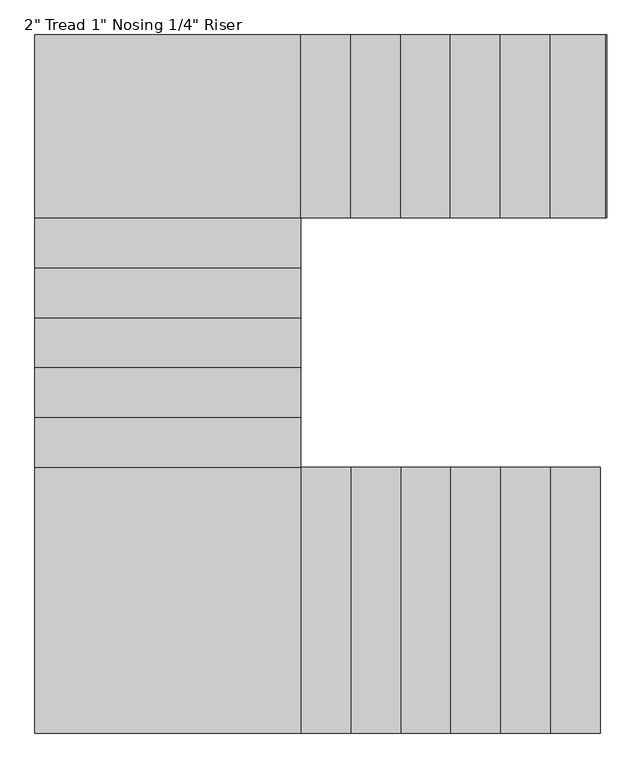
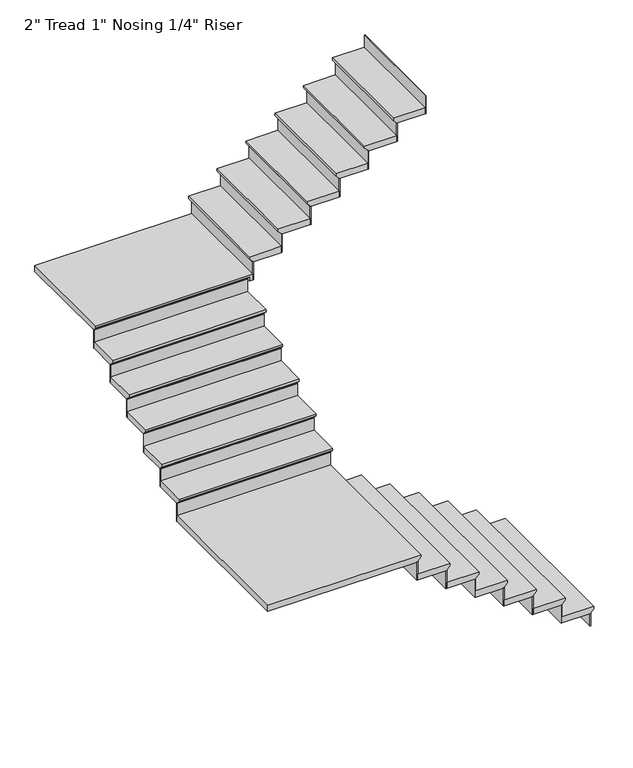
"""IFC4 building model written with IfcOpenShell, lengths in millimetres: stair flight geometry."""

from ifc_helpers import new_model, si_unit, origin, place, context, project, spatial, faceted_brep, source, transform, mapped, element, save


def stair_flight_f9fade56(model_context):
    return source(origin(), model_context, "Body", "Brep", [
        faceted_brep([(-2515.2117403, -5163.0426559, 15982.95), (-2515.2117403, -5163.0426559, 16002.0), (-2515.2117403, -6382.2426559, 16002.0), (-2515.2117403, -6382.2426559, 15982.95), (-2540.6117403, -5163.0426559, 15957.55), (-2540.6117403, -6382.2426559, 15957.55), (-2769.2117403, -5163.0426559, 16002.0), (-2769.2117403, -6382.2426559, 16002.0), (-2540.6117403, -6382.2426559, 15951.2), (-2769.2117403, -6382.2426559, 15951.2), (-2769.2117403, -5163.0426559, 15951.2), (-2540.6117403, -5163.0426559, 15951.2)], [[[0, 1, 2, 3]], [[4, 0, 3, 5]], [[2, 1, 6, 7]], [[8, 9, 10, 11]], [[2, 7, 9, 8, 5, 3]], [[8, 11, 4, 5]], [[6, 1, 0, 4, 11, 10]], [[7, 6, 10, 9]]]),
        faceted_brep([(-2540.6117403, -5163.0426559, 15951.2), (-2540.6117403, -5163.0426559, 15849.6), (-2546.9617403, -5163.0426559, 15849.6), (-2546.9617403, -5163.0426559, 15951.2), (-2540.6117403, -6382.2426559, 15951.2), (-2546.9617403, -6382.2426559, 15951.2), (-2546.9617403, -6382.2426559, 15849.6), (-2540.6117403, -6382.2426559, 15849.6)], [[[0, 1, 2, 3]], [[4, 5, 6, 7]], [[1, 0, 4, 7]], [[2, 1, 7, 6]], [[3, 2, 6, 5]], [[0, 3, 5, 4]]]),
        faceted_brep([(-2769.2117403, -5163.0426559, 16103.6), (-2769.2117403, -5163.0426559, 15951.2), (-2775.5617403, -5163.0426559, 15951.2), (-2775.5617403, -5163.0426559, 16103.6), (-2769.2117403, -6382.2426559, 16103.6), (-2775.5617403, -6382.2426559, 16103.6), (-2775.5617403, -6382.2426559, 15951.2), (-2769.2117403, -6382.2426559, 15951.2)], [[[0, 1, 2, 3]], [[4, 5, 6, 7]], [[1, 0, 4, 7]], [[2, 1, 7, 6]], [[3, 2, 6, 5]], [[0, 3, 5, 4]]]),
        faceted_brep([(-2743.8117403, -6382.2426559, 16154.4), (-2743.8117403, -5163.0426559, 16154.4), (-2997.8117403, -5163.0426559, 16154.4), (-2997.8117403, -6382.2426559, 16154.4), (-2769.2117403, -6382.2426559, 16103.6), (-2997.8117403, -6382.2426559, 16103.6), (-2997.8117403, -5163.0426559, 16103.6), (-2769.2117403, -5163.0426559, 16103.6), (-2769.2117403, -6382.2426559, 16109.95), (-2743.8117403, -6382.2426559, 16135.35), (-2769.2117403, -5163.0426559, 16109.95), (-2743.8117403, -5163.0426559, 16135.35)], [[[0, 1, 2, 3]], [[4, 5, 6, 7]], [[0, 3, 5, 4, 8, 9]], [[4, 7, 10, 8]], [[2, 1, 11, 10, 7, 6]], [[3, 2, 6, 5]], [[11, 1, 0, 9]], [[10, 11, 9, 8]]]),
        faceted_brep([(-2997.8117403, -5163.0426559, 16256.0), (-2997.8117403, -5163.0426559, 16103.6), (-3004.1617403, -5163.0426559, 16103.6), (-3004.1617403, -5163.0426559, 16256.0), (-2997.8117403, -6382.2426559, 16256.0), (-3004.1617403, -6382.2426559, 16256.0), (-3004.1617403, -6382.2426559, 16103.6), (-2997.8117403, -6382.2426559, 16103.6)], [[[0, 1, 2, 3]], [[4, 5, 6, 7]], [[1, 0, 4, 7]], [[2, 1, 7, 6]], [[3, 2, 6, 5]], [[0, 3, 5, 4]]]),
        faceted_brep([(-2972.4117403, -6382.2426559, 16306.8), (-2972.4117403, -5163.0426559, 16306.8), (-3226.4117403, -5163.0426559, 16306.8), (-3226.4117403, -6382.2426559, 16306.8), (-2997.8117403, -6382.2426559, 16256.0), (-3226.4117403, -6382.2426559, 16256.0), (-3226.4117403, -5163.0426559, 16256.0), (-2997.8117403, -5163.0426559, 16256.0), (-2997.8117403, -6382.2426559, 16262.35), (-2972.4117403, -6382.2426559, 16287.75), (-2997.8117403, -5163.0426559, 16262.35), (-2972.4117403, -5163.0426559, 16287.75)], [[[0, 1, 2, 3]], [[4, 5, 6, 7]], [[0, 3, 5, 4, 8, 9]], [[4, 7, 10, 8]], [[2, 1, 11, 10, 7, 6]], [[3, 2, 6, 5]], [[11, 1, 0, 9]], [[10, 11, 9, 8]]]),
        faceted_brep([(-3226.4117403, -5163.0426559, 16408.4), (-3226.4117403, -5163.0426559, 16256.0), (-3232.7617403, -5163.0426559, 16256.0), (-3232.7617403, -5163.0426559, 16408.4), (-3226.4117403, -6382.2426559, 16408.4), (-3232.7617403, -6382.2426559, 16408.4), (-3232.7617403, -6382.2426559, 16256.0), (-3226.4117403, -6382.2426559, 16256.0)], [[[0, 1, 2, 3]], [[4, 5, 6, 7]], [[1, 0, 4, 7]], [[2, 1, 7, 6]], [[3, 2, 6, 5]], [[0, 3, 5, 4]]]),
        faceted_brep([(-3201.0117403, -6382.2426559, 16459.2), (-3201.0117403, -5163.0426559, 16459.2), (-3455.0117403, -5163.0426559, 16459.2), (-3455.0117403, -6382.2426559, 16459.2), (-3226.4117403, -6382.2426559, 16408.4), (-3455.0117403, -6382.2426559, 16408.4), (-3455.0117403, -5163.0426559, 16408.4), (-3226.4117403, -5163.0426559, 16408.4), (-3226.4117403, -6382.2426559, 16414.75), (-3201.0117403, -6382.2426559, 16440.15), (-3226.4117403, -5163.0426559, 16414.75), (-3201.0117403, -5163.0426559, 16440.15)], [[[0, 1, 2, 3]], [[4, 5, 6, 7]], [[0, 3, 5, 4, 8, 9]], [[4, 7, 10, 8]], [[2, 1, 11, 10, 7, 6]], [[3, 2, 6, 5]], [[11, 1, 0, 9]], [[10, 11, 9, 8]]]),
        faceted_brep([(-3455.0117403, -5163.0426559, 16560.8), (-3455.0117403, -5163.0426559, 16408.4), (-3461.3617403, -5163.0426559, 16408.4), (-3461.3617403, -5163.0426559, 16560.8), (-3455.0117403, -6382.2426559, 16560.8), (-3461.3617403, -6382.2426559, 16560.8), (-3461.3617403, -6382.2426559, 16408.4), (-3455.0117403, -6382.2426559, 16408.4)], [[[0, 1, 2, 3]], [[4, 5, 6, 7]], [[1, 0, 4, 7]], [[2, 1, 7, 6]], [[3, 2, 6, 5]], [[0, 3, 5, 4]]]),
        faceted_brep([(-3429.6117403, -6382.2426559, 16611.6), (-3429.6117403, -5163.0426559, 16611.6), (-3683.6117403, -5163.0426559, 16611.6), (-3683.6117403, -6382.2426559, 16611.6), (-3455.0117403, -6382.2426559, 16560.8), (-3683.6117403, -6382.2426559, 16560.8), (-3683.6117403, -5163.0426559, 16560.8), (-3455.0117403, -5163.0426559, 16560.8), (-3455.0117403, -6382.2426559, 16567.15), (-3429.6117403, -6382.2426559, 16592.55), (-3455.0117403, -5163.0426559, 16567.15), (-3429.6117403, -5163.0426559, 16592.55)], [[[0, 1, 2, 3]], [[4, 5, 6, 7]], [[0, 3, 5, 4, 8, 9]], [[4, 7, 10, 8]], [[2, 1, 11, 10, 7, 6]], [[3, 2, 6, 5]], [[11, 1, 0, 9]], [[10, 11, 9, 8]]]),
        faceted_brep([(-3683.6117403, -5163.0426559, 16713.2), (-3683.6117403, -5163.0426559, 16560.8), (-3689.9617403, -5163.0426559, 16560.8), (-3689.9617403, -5163.0426559, 16713.2), (-3683.6117403, -6382.2426559, 16713.2), (-3689.9617403, -6382.2426559, 16713.2), (-3689.9617403, -6382.2426559, 16560.8), (-3683.6117403, -6382.2426559, 16560.8)], [[[0, 1, 2, 3]], [[4, 5, 6, 7]], [[1, 0, 4, 7]], [[2, 1, 7, 6]], [[3, 2, 6, 5]], [[0, 3, 5, 4]]]),
        faceted_brep([(-3658.2117403, -6382.2426559, 16764.0), (-3658.2117403, -5163.0426559, 16764.0), (-3912.2117403, -5163.0426559, 16764.0), (-3912.2117403, -6382.2426559, 16764.0), (-3683.6117403, -6382.2426559, 16713.2), (-3912.2117403, -6382.2426559, 16713.2), (-3912.2117403, -5163.0426559, 16713.2), (-3683.6117403, -5163.0426559, 16713.2), (-3683.6117403, -6382.2426559, 16719.55), (-3658.2117403, -6382.2426559, 16744.95), (-3683.6117403, -5163.0426559, 16719.55), (-3658.2117403, -5163.0426559, 16744.95)], [[[0, 1, 2, 3]], [[4, 5, 6, 7]], [[0, 3, 5, 4, 8, 9]], [[4, 7, 10, 8]], [[2, 1, 11, 10, 7, 6]], [[3, 2, 6, 5]], [[11, 1, 0, 9]], [[10, 11, 9, 8]]]),
        faceted_brep([(-3912.2117403, -5163.0426559, 16865.6), (-3912.2117403, -5163.0426559, 16713.2), (-3918.5617403, -5163.0426559, 16713.2), (-3918.5617403, -5163.0426559, 16865.6), (-3912.2117403, -6382.2426559, 16865.6), (-3918.5617403, -6382.2426559, 16865.6), (-3918.5617403, -6382.2426559, 16713.2), (-3912.2117403, -6382.2426559, 16713.2)], [[[0, 1, 2, 3]], [[4, 5, 6, 7]], [[1, 0, 4, 7]], [[2, 1, 7, 6]], [[3, 2, 6, 5]], [[0, 3, 5, 4]]]),
        faceted_brep([(-5106.0117403, -5137.6426559, 16916.4), (-5106.0117403, -6382.2426559, 16916.4), (-3886.8117403, -6382.2426559, 16916.4), (-3886.8117403, -5137.6426559, 16916.4), (-5106.0117403, -6382.2426559, 16865.6), (-5106.0117403, -5137.6426559, 16865.6), (-3886.8117403, -5137.6426559, 16865.6), (-3886.8117403, -5163.0426559, 16865.6), (-3912.2117403, -5163.0426559, 16865.6), (-3912.2117403, -6382.2426559, 16865.6), (-3912.2117403, -6382.2426559, 16871.95), (-3886.8117403, -6382.2426559, 16897.35), (-3912.2117403, -5163.0426559, 16871.95), (-3886.8117403, -5163.0426559, 16897.35)], [[[0, 1, 2, 3]], [[4, 5, 6, 7, 8, 9]], [[1, 0, 5, 4]], [[2, 1, 4, 9, 10, 11]], [[9, 8, 12, 10]], [[8, 7, 13, 12]], [[3, 2, 11, 13, 7, 6]], [[0, 3, 6, 5]], [[11, 10, 12, 13]]]),
        faceted_brep([(-3886.8117403, -5137.6426559, 17018.0), (-3886.8117403, -5137.6426559, 16865.6), (-3886.8117403, -5131.2926559, 16865.6), (-3886.8117403, -5131.2926559, 17018.0), (-5106.0117403, -5137.6426559, 17018.0), (-5106.0117403, -5131.2926559, 17018.0), (-5106.0117403, -5131.2926559, 16865.6), (-5106.0117403, -5137.6426559, 16865.6)], [[[0, 1, 2, 3]], [[4, 5, 6, 7]], [[1, 0, 4, 7]], [[2, 1, 7, 6]], [[3, 2, 6, 5]], [[0, 3, 5, 4]]]),
        faceted_brep([(-5106.0117403, -5163.0426559, 17068.8), (-3886.8117403, -5163.0426559, 17068.8), (-3886.8117403, -4909.0426559, 17068.8), (-5106.0117403, -4909.0426559, 17068.8), (-5106.0117403, -5137.6426559, 17018.0), (-5106.0117403, -4909.0426559, 17018.0), (-3886.8117403, -4909.0426559, 17018.0), (-3886.8117403, -5137.6426559, 17018.0), (-5106.0117403, -5137.6426559, 17024.35), (-5106.0117403, -5163.0426559, 17049.75), (-3886.8117403, -5137.6426559, 17024.35), (-3886.8117403, -5163.0426559, 17049.75)], [[[0, 1, 2, 3]], [[4, 5, 6, 7]], [[0, 3, 5, 4, 8, 9]], [[4, 7, 10, 8]], [[2, 1, 11, 10, 7, 6]], [[3, 2, 6, 5]], [[11, 1, 0, 9]], [[10, 11, 9, 8]]]),
        faceted_brep([(-3886.8117403, -4909.0426559, 17170.4), (-3886.8117403, -4909.0426559, 17018.0), (-3886.8117403, -4902.6926559, 17018.0), (-3886.8117403, -4902.6926559, 17170.4), (-5106.0117403, -4909.0426559, 17170.4), (-5106.0117403, -4902.6926559, 17170.4), (-5106.0117403, -4902.6926559, 17018.0), (-5106.0117403, -4909.0426559, 17018.0)], [[[0, 1, 2, 3]], [[4, 5, 6, 7]], [[1, 0, 4, 7]], [[2, 1, 7, 6]], [[3, 2, 6, 5]], [[0, 3, 5, 4]]]),
        faceted_brep([(-5106.0117403, -4934.4426559, 17221.2), (-3886.8117403, -4934.4426559, 17221.2), (-3886.8117403, -4680.4426559, 17221.2), (-5106.0117403, -4680.4426559, 17221.2), (-5106.0117403, -4909.0426559, 17170.4), (-5106.0117403, -4680.4426559, 17170.4), (-3886.8117403, -4680.4426559, 17170.4), (-3886.8117403, -4909.0426559, 17170.4), (-5106.0117403, -4909.0426559, 17176.75), (-5106.0117403, -4934.4426559, 17202.15), (-3886.8117403, -4909.0426559, 17176.75), (-3886.8117403, -4934.4426559, 17202.15)], [[[0, 1, 2, 3]], [[4, 5, 6, 7]], [[0, 3, 5, 4, 8, 9]], [[4, 7, 10, 8]], [[2, 1, 11, 10, 7, 6]], [[3, 2, 6, 5]], [[11, 1, 0, 9]], [[10, 11, 9, 8]]]),
        faceted_brep([(-3886.8117403, -4680.4426559, 17322.8), (-3886.8117403, -4680.4426559, 17170.4), (-3886.8117403, -4674.0926559, 17170.4), (-3886.8117403, -4674.0926559, 17322.8), (-5106.0117403, -4680.4426559, 17322.8), (-5106.0117403, -4674.0926559, 17322.8), (-5106.0117403, -4674.0926559, 17170.4), (-5106.0117403, -4680.4426559, 17170.4)], [[[0, 1, 2, 3]], [[4, 5, 6, 7]], [[1, 0, 4, 7]], [[2, 1, 7, 6]], [[3, 2, 6, 5]], [[0, 3, 5, 4]]]),
        faceted_brep([(-5106.0117403, -4705.8426559, 17373.6), (-3886.8117403, -4705.8426559, 17373.6), (-3886.8117403, -4451.8426559, 17373.6), (-5106.0117403, -4451.8426559, 17373.6), (-5106.0117403, -4680.4426559, 17322.8), (-5106.0117403, -4451.8426559, 17322.8), (-3886.8117403, -4451.8426559, 17322.8), (-3886.8117403, -4680.4426559, 17322.8), (-5106.0117403, -4680.4426559, 17329.15), (-5106.0117403, -4705.8426559, 17354.55), (-3886.8117403, -4680.4426559, 17329.15), (-3886.8117403, -4705.8426559, 17354.55)], [[[0, 1, 2, 3]], [[4, 5, 6, 7]], [[0, 3, 5, 4, 8, 9]], [[4, 7, 10, 8]], [[2, 1, 11, 10, 7, 6]], [[3, 2, 6, 5]], [[11, 1, 0, 9]], [[10, 11, 9, 8]]]),
        faceted_brep([(-3886.8117403, -4451.8426559, 17475.2), (-3886.8117403, -4451.8426559, 17322.8), (-3886.8117403, -4445.4926559, 17322.8), (-3886.8117403, -4445.4926559, 17475.2), (-5106.0117403, -4451.8426559, 17475.2), (-5106.0117403, -4445.4926559, 17475.2), (-5106.0117403, -4445.4926559, 17322.8), (-5106.0117403, -4451.8426559, 17322.8)], [[[0, 1, 2, 3]], [[4, 5, 6, 7]], [[1, 0, 4, 7]], [[2, 1, 7, 6]], [[3, 2, 6, 5]], [[0, 3, 5, 4]]]),
        faceted_brep([(-5106.0117403, -4477.2426559, 17526.0), (-3886.8117403, -4477.2426559, 17526.0), (-3886.8117403, -4223.2426559, 17526.0), (-5106.0117403, -4223.2426559, 17526.0), (-5106.0117403, -4451.8426559, 17475.2), (-5106.0117403, -4223.2426559, 17475.2), (-3886.8117403, -4223.2426559, 17475.2), (-3886.8117403, -4451.8426559, 17475.2), (-5106.0117403, -4451.8426559, 17481.55), (-5106.0117403, -4477.2426559, 17506.95), (-3886.8117403, -4451.8426559, 17481.55), (-3886.8117403, -4477.2426559, 17506.95)], [[[0, 1, 2, 3]], [[4, 5, 6, 7]], [[0, 3, 5, 4, 8, 9]], [[4, 7, 10, 8]], [[2, 1, 11, 10, 7, 6]], [[3, 2, 6, 5]], [[11, 1, 0, 9]], [[10, 11, 9, 8]]]),
        faceted_brep([(-3886.8117403, -4223.2426559, 17627.6), (-3886.8117403, -4223.2426559, 17475.2), (-3886.8117403, -4216.8926559, 17475.2), (-3886.8117403, -4216.8926559, 17627.6), (-5106.0117403, -4223.2426559, 17627.6), (-5106.0117403, -4216.8926559, 17627.6), (-5106.0117403, -4216.8926559, 17475.2), (-5106.0117403, -4223.2426559, 17475.2)], [[[0, 1, 2, 3]], [[4, 5, 6, 7]], [[1, 0, 4, 7]], [[2, 1, 7, 6]], [[3, 2, 6, 5]], [[0, 3, 5, 4]]]),
        faceted_brep([(-5106.0117403, -4248.6426559, 17678.4), (-3886.8117403, -4248.6426559, 17678.4), (-3886.8117403, -3994.6426559, 17678.4), (-5106.0117403, -3994.6426559, 17678.4), (-5106.0117403, -4223.2426559, 17627.6), (-5106.0117403, -3994.6426559, 17627.6), (-3886.8117403, -3994.6426559, 17627.6), (-3886.8117403, -4223.2426559, 17627.6), (-5106.0117403, -4223.2426559, 17633.95), (-5106.0117403, -4248.6426559, 17659.35), (-3886.8117403, -4223.2426559, 17633.95), (-3886.8117403, -4248.6426559, 17659.35)], [[[0, 1, 2, 3]], [[4, 5, 6, 7]], [[0, 3, 5, 4, 8, 9]], [[4, 7, 10, 8]], [[2, 1, 11, 10, 7, 6]], [[3, 2, 6, 5]], [[11, 1, 0, 9]], [[10, 11, 9, 8]]]),
        faceted_brep([(-3886.8117403, -3994.6426559, 17780.0), (-3886.8117403, -3994.6426559, 17627.6), (-3886.8117403, -3988.2926559, 17627.6), (-3886.8117403, -3988.2926559, 17780.0), (-5106.0117403, -3994.6426559, 17780.0), (-5106.0117403, -3988.2926559, 17780.0), (-5106.0117403, -3988.2926559, 17627.6), (-5106.0117403, -3994.6426559, 17627.6)], [[[0, 1, 2, 3]], [[4, 5, 6, 7]], [[1, 0, 4, 7]], [[2, 1, 7, 6]], [[3, 2, 6, 5]], [[0, 3, 5, 4]]]),
        faceted_brep([(-3861.4117403, -3181.8426559, 17830.8), (-5106.0117403, -3181.8426559, 17830.8), (-5106.0117403, -4020.0426559, 17830.8), (-3861.4117403, -4020.0426559, 17830.8), (-5106.0117403, -3181.8426559, 17780.0), (-3861.4117403, -3181.8426559, 17780.0), (-3861.4117403, -4020.0426559, 17780.0), (-3886.8117403, -4020.0426559, 17780.0), (-3886.8117403, -3994.6426559, 17780.0), (-5106.0117403, -3994.6426559, 17780.0), (-5106.0117403, -3994.6426559, 17786.35), (-5106.0117403, -4020.0426559, 17811.75), (-3886.8117403, -3994.6426559, 17786.35), (-3886.8117403, -4020.0426559, 17811.75)], [[[0, 1, 2, 3]], [[4, 5, 6, 7, 8, 9]], [[1, 0, 5, 4]], [[2, 1, 4, 9, 10, 11]], [[9, 8, 12, 10]], [[8, 7, 13, 12]], [[3, 2, 11, 13, 7, 6]], [[0, 3, 6, 5]], [[11, 10, 12, 13]]]),
        faceted_brep([(-3861.4117403, -4020.0426559, 17932.4), (-3861.4117403, -4020.0426559, 17780.0), (-3855.0617403, -4020.0426559, 17780.0), (-3855.0617403, -4020.0426559, 17932.4), (-3861.4117403, -3181.8426559, 17932.4), (-3855.0617403, -3181.8426559, 17932.4), (-3855.0617403, -3181.8426559, 17780.0), (-3861.4117403, -3181.8426559, 17780.0)], [[[0, 1, 2, 3]], [[4, 5, 6, 7]], [[1, 0, 4, 7]], [[2, 1, 7, 6]], [[3, 2, 6, 5]], [[0, 3, 5, 4]]]),
        faceted_brep([(-3886.8117403, -3181.8426559, 17983.2), (-3886.8117403, -4020.0426559, 17983.2), (-3632.8117403, -4020.0426559, 17983.2), (-3632.8117403, -3181.8426559, 17983.2), (-3861.4117403, -3181.8426559, 17932.4), (-3632.8117403, -3181.8426559, 17932.4), (-3632.8117403, -4020.0426559, 17932.4), (-3861.4117403, -4020.0426559, 17932.4), (-3861.4117403, -3181.8426559, 17938.75), (-3886.8117403, -3181.8426559, 17964.15), (-3861.4117403, -4020.0426559, 17938.75), (-3886.8117403, -4020.0426559, 17964.15)], [[[0, 1, 2, 3]], [[4, 5, 6, 7]], [[0, 3, 5, 4, 8, 9]], [[4, 7, 10, 8]], [[2, 1, 11, 10, 7, 6]], [[3, 2, 6, 5]], [[11, 1, 0, 9]], [[10, 11, 9, 8]]]),
        faceted_brep([(-3632.8117403, -4020.0426559, 18084.8), (-3632.8117403, -4020.0426559, 17932.4), (-3626.4617403, -4020.0426559, 17932.4), (-3626.4617403, -4020.0426559, 18084.8), (-3632.8117403, -3181.8426559, 18084.8), (-3626.4617403, -3181.8426559, 18084.8), (-3626.4617403, -3181.8426559, 17932.4), (-3632.8117403, -3181.8426559, 17932.4)], [[[0, 1, 2, 3]], [[4, 5, 6, 7]], [[1, 0, 4, 7]], [[2, 1, 7, 6]], [[3, 2, 6, 5]], [[0, 3, 5, 4]]]),
        faceted_brep([(-3658.2117403, -3181.8426559, 18135.6), (-3658.2117403, -4020.0426559, 18135.6), (-3404.2117403, -4020.0426559, 18135.6), (-3404.2117403, -3181.8426559, 18135.6), (-3632.8117403, -3181.8426559, 18084.8), (-3404.2117403, -3181.8426559, 18084.8), (-3404.2117403, -4020.0426559, 18084.8), (-3632.8117403, -4020.0426559, 18084.8), (-3632.8117403, -3181.8426559, 18091.15), (-3658.2117403, -3181.8426559, 18116.55), (-3632.8117403, -4020.0426559, 18091.15), (-3658.2117403, -4020.0426559, 18116.55)], [[[0, 1, 2, 3]], [[4, 5, 6, 7]], [[0, 3, 5, 4, 8, 9]], [[4, 7, 10, 8]], [[2, 1, 11, 10, 7, 6]], [[3, 2, 6, 5]], [[11, 1, 0, 9]], [[10, 11, 9, 8]]]),
        faceted_brep([(-3404.2117403, -4020.0426559, 18237.2), (-3404.2117403, -4020.0426559, 18084.8), (-3397.8617403, -4020.0426559, 18084.8), (-3397.8617403, -4020.0426559, 18237.2), (-3404.2117403, -3181.8426559, 18237.2), (-3397.8617403, -3181.8426559, 18237.2), (-3397.8617403, -3181.8426559, 18084.8), (-3404.2117403, -3181.8426559, 18084.8)], [[[0, 1, 2, 3]], [[4, 5, 6, 7]], [[1, 0, 4, 7]], [[2, 1, 7, 6]], [[3, 2, 6, 5]], [[0, 3, 5, 4]]]),
        faceted_brep([(-3429.6117403, -3181.8426559, 18288.0), (-3429.6117403, -4020.0426559, 18288.0), (-3175.6117403, -4020.0426559, 18288.0), (-3175.6117403, -3181.8426559, 18288.0), (-3404.2117403, -3181.8426559, 18237.2), (-3175.6117403, -3181.8426559, 18237.2), (-3175.6117403, -4020.0426559, 18237.2), (-3404.2117403, -4020.0426559, 18237.2), (-3404.2117403, -3181.8426559, 18243.55), (-3429.6117403, -3181.8426559, 18268.95), (-3404.2117403, -4020.0426559, 18243.55), (-3429.6117403, -4020.0426559, 18268.95)], [[[0, 1, 2, 3]], [[4, 5, 6, 7]], [[0, 3, 5, 4, 8, 9]], [[4, 7, 10, 8]], [[2, 1, 11, 10, 7, 6]], [[3, 2, 6, 5]], [[11, 1, 0, 9]], [[10, 11, 9, 8]]]),
        faceted_brep([(-3175.6117403, -4020.0426559, 18389.6), (-3175.6117403, -4020.0426559, 18237.2), (-3169.2617403, -4020.0426559, 18237.2), (-3169.2617403, -4020.0426559, 18389.6), (-3175.6117403, -3181.8426559, 18389.6), (-3169.2617403, -3181.8426559, 18389.6), (-3169.2617403, -3181.8426559, 18237.2), (-3175.6117403, -3181.8426559, 18237.2)], [[[0, 1, 2, 3]], [[4, 5, 6, 7]], [[1, 0, 4, 7]], [[2, 1, 7, 6]], [[3, 2, 6, 5]], [[0, 3, 5, 4]]]),
        faceted_brep([(-3201.0117403, -3181.8426559, 18440.4), (-3201.0117403, -4020.0426559, 18440.4), (-2947.0117403, -4020.0426559, 18440.4), (-2947.0117403, -3181.8426559, 18440.4), (-3175.6117403, -3181.8426559, 18389.6), (-2947.0117403, -3181.8426559, 18389.6), (-2947.0117403, -4020.0426559, 18389.6), (-3175.6117403, -4020.0426559, 18389.6), (-3175.6117403, -3181.8426559, 18395.95), (-3201.0117403, -3181.8426559, 18421.35), (-3175.6117403, -4020.0426559, 18395.95), (-3201.0117403, -4020.0426559, 18421.35)], [[[0, 1, 2, 3]], [[4, 5, 6, 7]], [[0, 3, 5, 4, 8, 9]], [[4, 7, 10, 8]], [[2, 1, 11, 10, 7, 6]], [[3, 2, 6, 5]], [[11, 1, 0, 9]], [[10, 11, 9, 8]]]),
        faceted_brep([(-2947.0117403, -4020.0426559, 18542.0), (-2947.0117403, -4020.0426559, 18389.6), (-2940.6617403, -4020.0426559, 18389.6), (-2940.6617403, -4020.0426559, 18542.0), (-2947.0117403, -3181.8426559, 18542.0), (-2940.6617403, -3181.8426559, 18542.0), (-2940.6617403, -3181.8426559, 18389.6), (-2947.0117403, -3181.8426559, 18389.6)], [[[0, 1, 2, 3]], [[4, 5, 6, 7]], [[1, 0, 4, 7]], [[2, 1, 7, 6]], [[3, 2, 6, 5]], [[0, 3, 5, 4]]]),
        faceted_brep([(-2972.4117403, -3181.8426559, 18592.8), (-2972.4117403, -4020.0426559, 18592.8), (-2718.4117403, -4020.0426559, 18592.8), (-2718.4117403, -3181.8426559, 18592.8), (-2947.0117403, -3181.8426559, 18542.0), (-2718.4117403, -3181.8426559, 18542.0), (-2718.4117403, -4020.0426559, 18542.0), (-2947.0117403, -4020.0426559, 18542.0), (-2947.0117403, -3181.8426559, 18548.35), (-2972.4117403, -3181.8426559, 18573.75), (-2947.0117403, -4020.0426559, 18548.35), (-2972.4117403, -4020.0426559, 18573.75)], [[[0, 1, 2, 3]], [[4, 5, 6, 7]], [[0, 3, 5, 4, 8, 9]], [[4, 7, 10, 8]], [[2, 1, 11, 10, 7, 6]], [[3, 2, 6, 5]], [[11, 1, 0, 9]], [[10, 11, 9, 8]]]),
        faceted_brep([(-2718.4117403, -4020.0426559, 18694.4), (-2718.4117403, -4020.0426559, 18542.0), (-2712.0617403, -4020.0426559, 18542.0), (-2712.0617403, -4020.0426559, 18694.4), (-2718.4117403, -3181.8426559, 18694.4), (-2712.0617403, -3181.8426559, 18694.4), (-2712.0617403, -3181.8426559, 18542.0), (-2718.4117403, -3181.8426559, 18542.0)], [[[0, 1, 2, 3]], [[4, 5, 6, 7]], [[1, 0, 4, 7]], [[2, 1, 7, 6]], [[3, 2, 6, 5]], [[0, 3, 5, 4]]]),
        faceted_brep([(-2489.8117403, -4020.0426559, 18846.8), (-2489.8117403, -4020.0426559, 18694.4), (-2483.4617403, -4020.0426559, 18694.4), (-2483.4617403, -4020.0426559, 18846.8), (-2489.8117403, -3181.8426559, 18846.8), (-2483.4617403, -3181.8426559, 18846.8), (-2483.4617403, -3181.8426559, 18694.4), (-2489.8117403, -3181.8426559, 18694.4)], [[[0, 1, 2, 3]], [[4, 5, 6, 7]], [[1, 0, 4, 7]], [[2, 1, 7, 6]], [[3, 2, 6, 5]], [[0, 3, 5, 4]]]),
        faceted_brep([(-2743.8117403, -3181.8426559, 18745.2), (-2743.8117403, -4020.0426559, 18745.2), (-2489.8117403, -4020.0426559, 18745.2), (-2489.8117403, -3181.8426559, 18745.2), (-2718.4117403, -3181.8426559, 18694.4), (-2489.8117403, -3181.8426559, 18694.4), (-2489.8117403, -4020.0426559, 18694.4), (-2718.4117403, -4020.0426559, 18694.4), (-2718.4117403, -3181.8426559, 18700.75), (-2743.8117403, -3181.8426559, 18726.15), (-2718.4117403, -4020.0426559, 18700.75), (-2743.8117403, -4020.0426559, 18726.15)], [[[0, 1, 2, 3]], [[4, 5, 6, 7]], [[0, 3, 5, 4, 8, 9]], [[4, 7, 10, 8]], [[2, 1, 11, 10, 7, 6]], [[3, 2, 6, 5]], [[11, 1, 0, 9]], [[10, 11, 9, 8]]]),
    ])


if __name__ == "__main__":
    model = new_model("IFC4")
    model_context = context("Model", 3, world=origin())
    ifc_project = project(units=[si_unit("LENGTHUNIT", "METRE", prefix="MILLI")], contexts=[model_context])
    site = spatial("IfcSite", under=ifc_project)
    building = spatial("IfcBuilding", under=site)
    placement = place(None, origin())
    stair_flight_shape = stair_flight_f9fade56(model_context)
    element("IfcStairFlight", 1, ObjectType="2\" Tread 1\" Nosing 1/4\" Riser", at=placement, inside=building, context=model_context, shape_type="MappedRepresentation", body=[
        mapped(stair_flight_shape, transform((0.0, 0.0, 0.0), x_axis=(1.0, 0.0, 0.0), y_axis=(0.0, 1.0, 0.0), z_axis=(0.0, 0.0, 1.0))),
    ])
    save(model, "model.ifc")

# Revit data of these elements
# Element 1 (IfcStairFlight, "2\" Tread 1\" Nosing 1/4\" Riser")
#   Materials on its faces: "Wood Planks"
# Materials
#   "Wood Planks": class "Wood", colour RGB 193 160 115, transparency 0, Description = "Physical material.", Cost = 0
